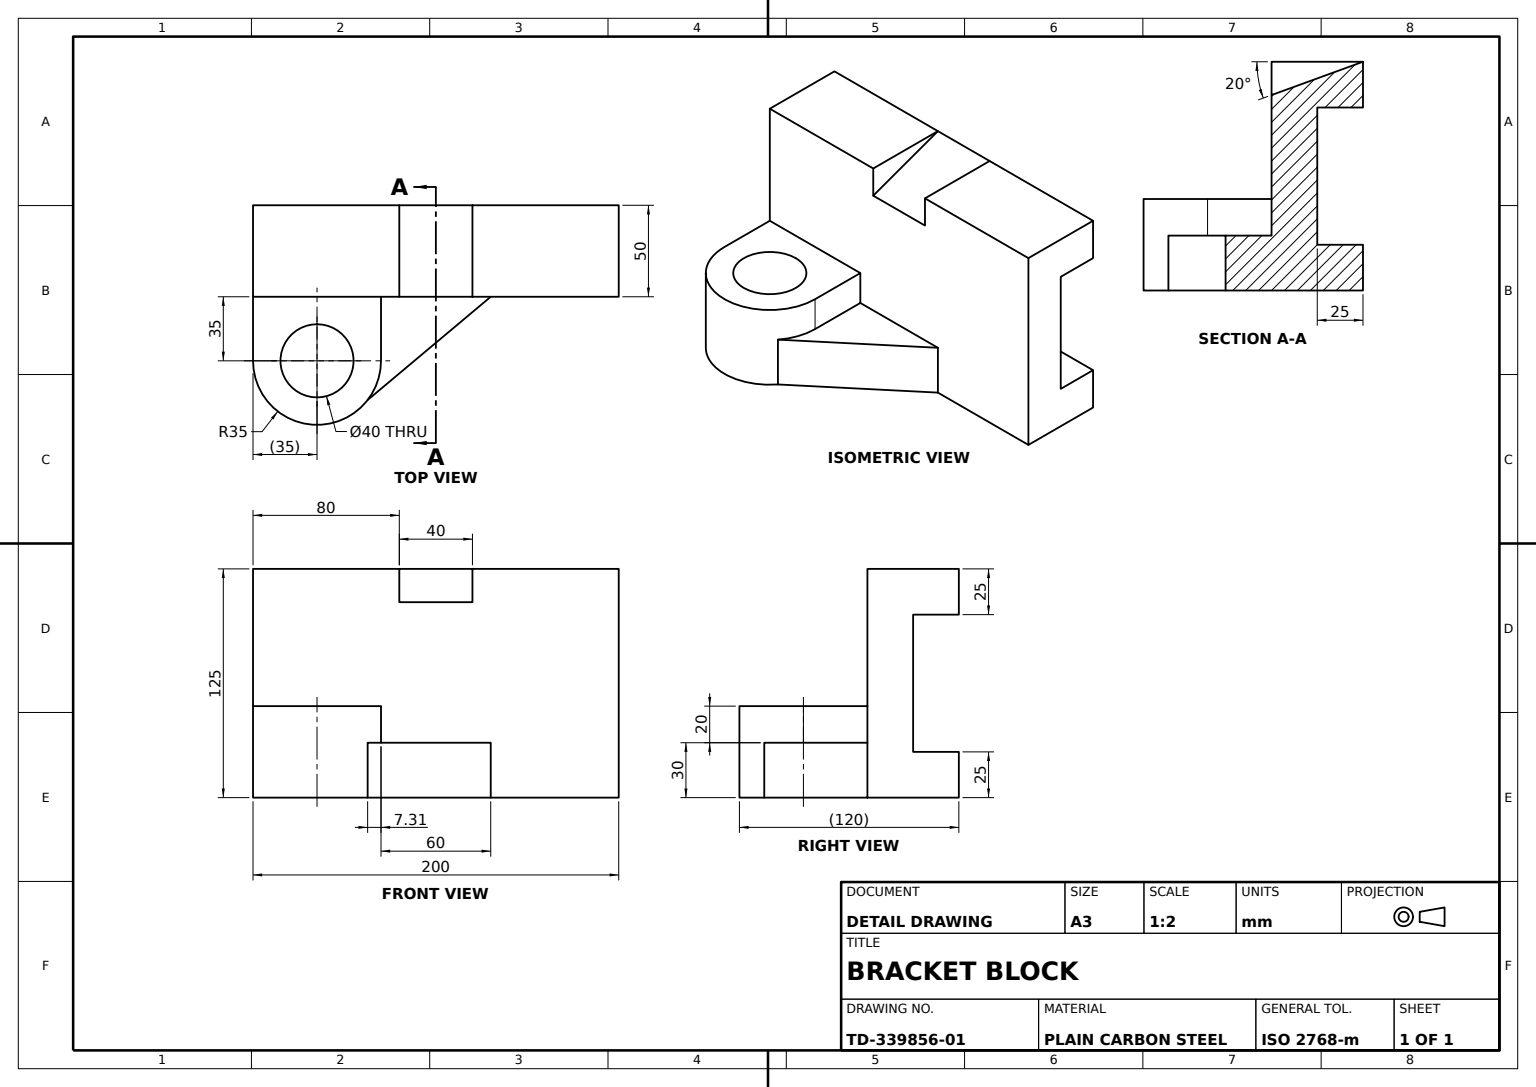
SolidWorks part; units mm, degrees
material "Plain Carbon Steel"
ref_plane "Front Plane" through (0, 0, 0) normal (0, 0, 1) x (1, 0, 0)
ref_plane "Top Plane" through (0, 0, 0) normal (0, 1, 0) x (1, 0, 0)
ref_plane "Right Plane" through (0, 0, 0) normal (1, 0, 0) x (0, 0, -1)
sketch "Base Block Sketch" plane through (0, 0, 0) normal (0, 0, 1) x (1, 0, 0)
  line L0 (0, 0) -> (0, -125)
  line L1 (0, -125) -> (200, -125)
  line L2 (200, -125) -> (200, 0)
  line L3 (200, 0) -> (0, 0)
  dimension "D1" = 200
  dimension "D2" = 125
extrude "Base Block" add sketch "Base Block Sketch" along normal blind 50
sketch "Upper Block Sketch" plane through (0, 0, 0) normal (0, 1, 0) x (1, 0, 0)
  line L0 (0, 0) -> (70, 0)
  line L1 (200, 0) -> (0, 0) construction
  line L2 (70, 0) -> (70, 35)
  line L4 (0, 35) -> (0, 0)
  arc A0 (70, 35) -> (0, 35) centre (35, 35) ccw
  dimension "D1" = 35
extrude "Upper Block" add sketch "Upper Block Sketch" against normal blind 50
sketch "Lug Sketch" plane through (0, 0, 0) normal (0, 1, 0) x (1, 0, 0)
  line L0 (200, 0) -> (130, 0)
  line L1 (200, 0) -> (70, 0) construction
  line L2 (130, 0) -> (62.6861, 56.4122)
  line L4 (70, 35) -> (70, 0)
  line L5 (70, 0) -> (130, 0)
  line L6 (70, 0) -> (70, 35) construction
  arc A0 (70, 35) -> (0, 35) centre (35, 35) ccw construction
  arc A1 (70, 35) -> (62.6861, 56.4122) centre (35, 35) ccw
  line M1 (200, 0) -> (70, 0)
  line M2 (70, 0) -> (70, 35)
  arc M3 (70, 35) -> (0, 35) centre (35, 35) ccw
  dimension "D1" = 60
  dimension "D2" = 7.3139
extrude "Lug Boss" add sketch "Lug Sketch" against normal blind 30 contours L2 M1 M3 M2
sketch "Lug Bore Sketch" plane through (0, -50, 0) normal (0, -1, 0) x (1, 0, 0)
  line L0 (35, 0) -> (35, -35)
  line L1 (0, 0) -> (70, 0) construction
  circle A0 centre (35, -35) radius 20
  dimension "D1" = 40
  dimension "D2" = 35
extrude "Lug Bore" cut sketch "Lug Bore Sketch" against normal blind 50
sketch "Channel Sketch" plane through (200, 0, 0) normal (1, 0, 0) x (0, 0, -1)
  line L0 (-50, -62.5) -> (-50, -25)
  line L1 (-50, -125) -> (-50, 0) construction
  line L2 (-50, -25) -> (-25, -25)
  line L3 (-25, -25) -> (-25, -100)
  line L4 (-25, -100) -> (-50, -100)
  line L5 (-50, -100) -> (-50, -62.5)
  line L6 (0, -125) -> (0, 0) construction
  line L7 (-50, 0) -> (0, 0) construction
  dimension "D1" = 25
  dimension "D2" = 25
extrude "Channel Cut" cut sketch "Channel Sketch" against normal blind 200
sketch "Corner Trim Sketch" plane through (200, 0, 0) normal (1, 0, 0) x (0, 0, -1)
  line L0 (-50, -125) -> (0.0509, -106.783)
  line L1 (0.0509, -106.783) -> (0, -125)
  line L2 (-50, -100) -> (-25, -100) construction
  line L3 (-25, -100) -> (-25, -25) construction
  line L4 (0, -125) -> (-50, -125)
  dimension "D1" = 25.0509
  dimension "D2" = 25
  dimension "D3" = 6.783
extrude "Corner Trim Cut" cut sketch "Corner Trim Sketch" against normal blind 200
sketch "Taper Fill 1 Sketch" plane through (200, 0, 0) normal (1, 0, 0) x (0, 0, -1)
  line L0 (-50, -125) -> (0, -106.8015)
  line L1 (0, -106.8015) -> (0, -125)
  line L2 (0, -125) -> (-50, -125)
extrude "Taper Fill 1" add sketch "Taper Fill 1 Sketch" against normal blind 80
sketch "Taper Fill 2 Sketch" plane through (0, 0, 0) normal (-1, 0, 0) x (0, 0, 1)
  line L0 (0, -106.8015) -> (50, -125)
  line L1 (50, -125) -> (0, -125)
  line L2 (0, -125) -> (0, -106.8015)
extrude "Taper Fill 2" add sketch "Taper Fill 2 Sketch" against normal blind 80
